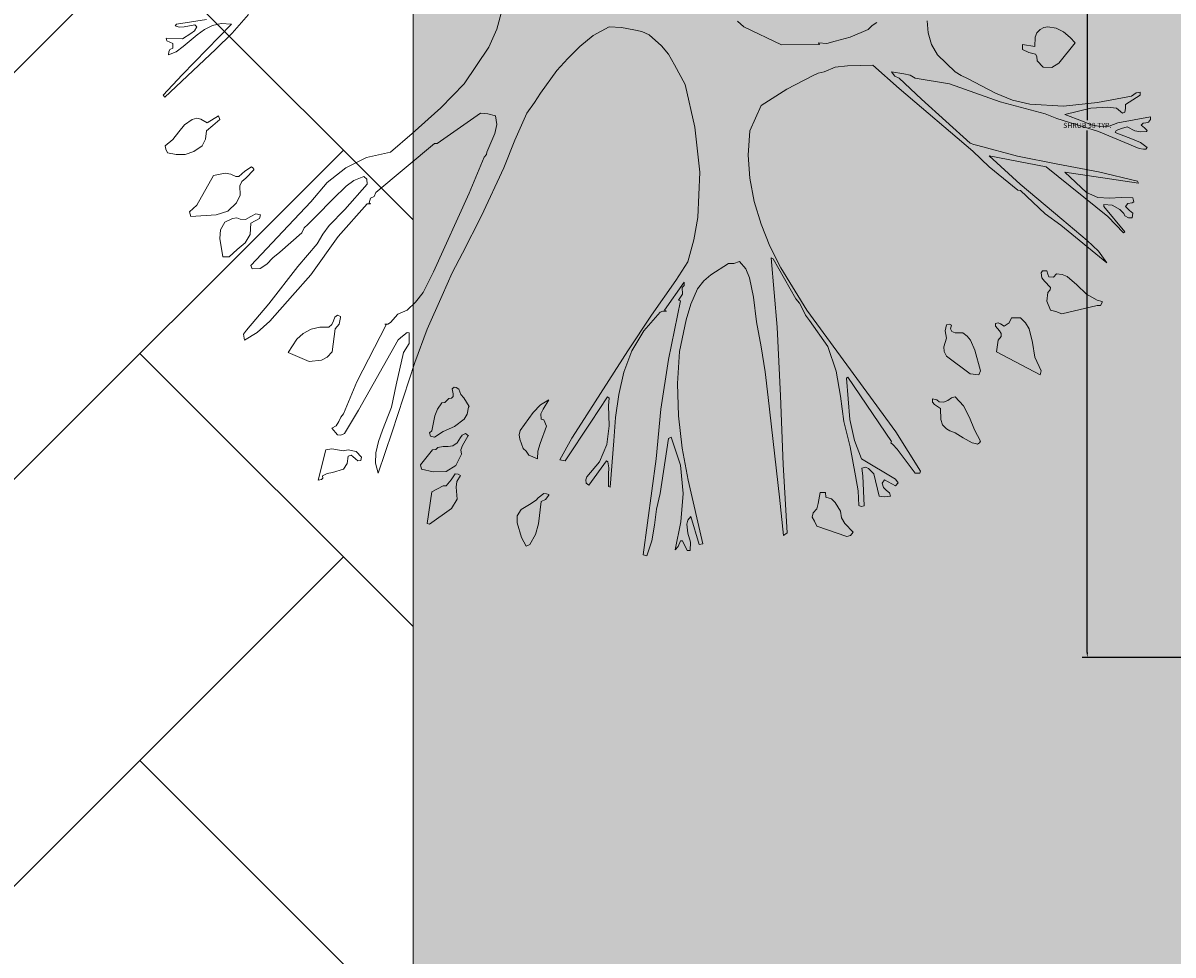
# Model space of a CAD drawing. Units: inches. Extents: x 84 to 1044, y -280 to 906.
# Tile 9 of 105: x 441 to 482, y -79 to -46. Entities that reach past the tile are written whole.
import ezdxf

# ---------------------------------------------------------------- set-up
doc = ezdxf.new("R2010")
doc.units = ezdxf.units.IN
for name, color, linetype, lineweight in [('A-ANNO-DIMS', 2, 'Continuous', 18), ('L-HRDS', 32, 'Continuous', 18), ('L-PLNT', 114, 'Continuous', 15)]:
    doc.layers.add(name, color=color, linetype=linetype, lineweight=lineweight)
doc.layers.add('L-PLNT-PATT', color=9, linetype='Continuous', lineweight=9, true_color=0xafd9aa)
doc.layers.add('L-PRKG-PATT', color=35, linetype='Continuous', lineweight=9, true_color=0x947764)
doc.styles.get("Standard").update_dxf_attribs({"font": 'arial.ttf'})
doc.dimstyles.get("Standard").update_dxf_attribs({"dimtxt": 0.18, "dimasz": 0.18, "dimexe": 0.18, "dimexo": 0.0625, "dimgap": 0.09, "dimtad": 0, "dimtih": 1, "dimtoh": 1, "dimdec": 4, "dimzin": 0, "dimdsep": 46, "dimtxsty": 'Standard', "dimcen": 0.09, "dimadec": 0, "dimazin": 0, "dimtfac": 1, "dimtdec": 4, "dimtofl": 0, "dimtmove": 0, "dimatfit": 3, "dimfxl": 1, "dimtolj": 1, "dimtzin": 0, "dimarcsym": 0})

# ---------------------------------------------------------------- blocks, each defined once
blk = doc.blocks.new('A$C37E508DF')
for p, q in [((0.9287, 0.7825), (0.936, 0.7542)), ((1.3151, 0.7487), (1.2919, 0.7752)), ((0.1351, 0.7559), (0.1471, 0.7577)), ((0.1471, 0.7577), (0.1527, 0.7568)), ((0.3186, 0.7491), (0.3199, 0.7662)), ((0.3919, 0.7641), (0.3988, 0.7598)), ((0.3988, 0.7598), (0.4043, 0.7538)), ((0.5287, 0.7319), (0.5823, 0.7577)), ((0.5823, 0.7577), (0.5913, 0.7658)), ((0.7752, 0.7577), (0.7577, 0.7568)), ((0.798, 0.7452), (0.7752, 0.7577)), ((1.3309, 0.7624), (1.3164, 0.7615)), ((1.3164, 0.7615), (1.3871, 0.6891)), ((1.3434, 0.7598), (1.3309, 0.7624)), ((1.355, 0.7538), (1.3434, 0.7598)), ((1.352, 0.7684), (1.3948, 0.7615)), ((1.3687, 0.7607), (1.3657, 0.7577)), ((1.3657, 0.7577), (1.3691, 0.7521)), ((1.3841, 0.7577), (1.3687, 0.7607)), ((1.3914, 0.7572), (1.3841, 0.7577)), ((1.397, 0.759), (1.3914, 0.7572)), ((1.3948, 0.7615), (1.397, 0.759)), ((0.1081, 0.7349), (0.1153, 0.7427)), ((0.1153, 0.7427), (0.1244, 0.7504)), ((0.1244, 0.7504), (0.1351, 0.7559)), ((0.1527, 0.7568), (0.1578, 0.7538)), ((0.1578, 0.7538), (0.1629, 0.7491)), ((0.1629, 0.7491), (0.1651, 0.7431)), ((0.1651, 0.7431), (0.1655, 0.7298)), ((0.3139, 0.7324), (0.3186, 0.7491)), ((0.4043, 0.7538), (0.4301, 0.7431)), ((0.4301, 0.7431), (0.4515, 0.7371)), ((0.7182, 0.7461), (0.7002, 0.7307)), ((0.7285, 0.7512), (0.7182, 0.7461)), ((0.7401, 0.7534), (0.7285, 0.7512)), ((0.7577, 0.7568), (0.7401, 0.7534)), ((0.8173, 0.7298), (0.798, 0.7452)), ((0.936, 0.7542), (0.9476, 0.7285)), ((1.3391, 0.7255), (1.3151, 0.7487)), ((1.3653, 0.7461), (1.355, 0.7538)), ((1.3854, 0.7294), (1.3653, 0.7461)), ((1.3691, 0.7521), (1.3743, 0.7482)), ((1.3743, 0.7482), (1.3863, 0.7405)), ((1.3863, 0.7405), (1.4099, 0.7414)), ((1.4099, 0.7414), (1.4086, 0.7375)), ((0.1312, 0.7058), (0.1081, 0.7349)), ((0.1655, 0.7298), (0.1831, 0.7324)), ((0.1831, 0.7255), (0.1741, 0.7208)), ((0.1831, 0.7324), (0.1831, 0.7255)), ((0.3049, 0.7178), (0.3139, 0.7324)), ((0.4515, 0.7371), (0.4635, 0.7341)), ((0.4635, 0.7341), (0.4755, 0.7349)), ((0.4755, 0.7349), (0.4742, 0.7324)), ((0.4742, 0.7324), (0.5287, 0.7319)), ((0.7002, 0.7307), (0.6903, 0.7186)), ((0.8344, 0.7122), (0.8173, 0.7298)), ((0.9476, 0.7285), (0.9828, 0.6762)), ((1.4116, 0.6569), (1.3391, 0.7255)), ((1.3953, 0.7221), (1.3854, 0.7294)), ((1.4086, 0.7375), (1.4004, 0.7337)), ((1.4004, 0.7337), (1.4004, 0.7272)), ((1.4004, 0.7272), (1.4047, 0.7255)), ((1.4047, 0.7255), (1.406, 0.7221)), ((0.1621, 0.7092), (0.1539, 0.7002)), ((0.1629, 0.7152), (0.1621, 0.7092)), ((0.1646, 0.7186), (0.1629, 0.7152)), ((0.1741, 0.7208), (0.1646, 0.7186)), ((0.28, 0.6933), (0.3049, 0.7178)), ((0.6903, 0.7186), (0.6818, 0.7032)), ((0.8503, 0.6951), (0.8344, 0.7122)), ((1.4064, 0.7178), (1.3953, 0.7221)), ((1.406, 0.7221), (1.4064, 0.7178)), ((0.1415, 0.6994), (0.1312, 0.7058)), ((0.1539, 0.7002), (0.1415, 0.6994)), ((0.271, 0.6882), (0.28, 0.6933)), ((0.3709, 0.6933), (0.3533, 0.6903)), ((0.3975, 0.7028), (0.3598, 0.6693)), ((0.3662, 0.6873), (0.3709, 0.6933)), ((0.4339, 0.7019), (0.3975, 0.7028)), ((0.4515, 0.7002), (0.4339, 0.7019)), ((0.4674, 0.6933), (0.4515, 0.7002)), ((0.476, 0.6912), (0.4674, 0.6933)), ((0.6818, 0.7032), (0.6667, 0.6749)), ((0.8739, 0.6629), (0.8503, 0.6951)), ((0.2877, 0.6762), (0.2152, 0.6505)), ((0.2221, 0.6625), (0.262, 0.6839)), ((0.262, 0.6839), (0.271, 0.6882)), ((0.337, 0.6843), (0.2877, 0.6762)), ((0.328, 0.6543), (0.3598, 0.6843)), ((0.3443, 0.6886), (0.337, 0.6843)), ((0.3533, 0.6903), (0.3443, 0.6886)), ((0.3598, 0.6843), (0.3662, 0.6873)), ((0.4832, 0.6878), (0.476, 0.6912)), ((0.521, 0.6685), (0.4832, 0.6878)), ((0.9828, 0.6762), (1.0162, 0.6415)), ((1.3871, 0.6891), (1.4141, 0.6599)), ((0.0146, 0.6599), (0.0146, 0.6642)), ((0.0146, 0.6642), (0.0206, 0.6633)), ((0.036, 0.6466), (0.0146, 0.6599)), ((0.0206, 0.6633), (0.0274, 0.6586)), ((0.1977, 0.6526), (0.2221, 0.6625)), ((0.3598, 0.6693), (0.2543, 0.5797)), ((0.5578, 0.6449), (0.521, 0.6685)), ((0.6667, 0.6749), (0.6526, 0.614)), ((0.8824, 0.6492), (0.8739, 0.6629)), ((1.4141, 0.6599), (1.4116, 0.6569)), ((0.0274, 0.6586), (0.0759, 0.6492)), ((0.0356, 0.6406), (0.036, 0.6466)), ((0.0609, 0.6428), (0.0489, 0.641)), ((0.0853, 0.641), (0.0609, 0.6428)), ((0.0759, 0.6492), (0.1244, 0.644)), ((0.1244, 0.644), (0.1728, 0.647)), ((0.2152, 0.6505), (0.1509, 0.6333)), ((0.1728, 0.647), (0.1977, 0.6526)), ((0.2581, 0.5913), (0.328, 0.6543)), ((0.5737, 0.6089), (0.5578, 0.6449)), ((0.8932, 0.6342), (0.8824, 0.6492)), ((0, 0.629), (0.0467, 0.62)), ((0, 0.6252), (0, 0.629)), ((0.0369, 0.6355), (0.0356, 0.6406)), ((0.0399, 0.6342), (0.0369, 0.6355)), ((0.0489, 0.641), (0.0399, 0.6342)), ((0.1226, 0.632), (0.0853, 0.641)), ((0.0973, 0.6226), (0.1226, 0.632)), ((0.1342, 0.6265), (0.1175, 0.6213)), ((0.1509, 0.6333), (0.1342, 0.6265)), ((0.9103, 0.5956), (0.8932, 0.6342)), ((0.9382, 0.6303), (0.936, 0.6179)), ((0.9493, 0.6333), (0.9382, 0.6303)), ((0.9596, 0.6342), (0.9493, 0.6333)), ((1.0218, 0.5904), (0.9596, 0.6342)), ((1.0162, 0.6415), (1.0574, 0.605)), ((1.3327, 0.6252), (1.3348, 0.6303)), ((1.3348, 0.6303), (1.3511, 0.62)), ((1.3601, 0.6256), (1.3661, 0.6269)), ((1.3661, 0.6269), (1.3725, 0.6252)), ((0.003, 0.6213), (0, 0.6252)), ((0.0069, 0.6204), (0.003, 0.6213)), ((0.0047, 0.6093), (0.0086, 0.6132)), ((0.0107, 0.6196), (0.0069, 0.6204)), ((0.0086, 0.6132), (0.0133, 0.617)), ((0.0133, 0.617), (0.0107, 0.6196)), ((0.0334, 0.6145), (0.0223, 0.6089)), ((0.0416, 0.6119), (0.0334, 0.6145)), ((0.0493, 0.6093), (0.0416, 0.6119)), ((0.0467, 0.62), (0.0592, 0.6153)), ((0.0592, 0.6153), (0.072, 0.6149)), ((0.072, 0.6149), (0.0849, 0.6175)), ((0.1175, 0.6213), (0.0746, 0.6076)), ((0.0849, 0.6175), (0.0973, 0.6226)), ((0.6526, 0.614), (0.6457, 0.5497)), ((0.936, 0.6179), (0.939, 0.605)), ((1.343, 0.6162), (1.3327, 0.6252)), ((1.352, 0.6089), (1.343, 0.6162)), ((1.3511, 0.62), (1.3601, 0.6256)), ((1.3725, 0.6252), (1.3837, 0.6175)), ((1.3837, 0.6175), (1.3918, 0.6072)), ((0.0056, 0.6076), (0.0047, 0.6093)), ((0.0141, 0.6072), (0.0056, 0.6076)), ((0.0223, 0.6089), (0.0141, 0.6072)), ((0.0141, 0.5921), (0.0257, 0.5969)), ((0.0746, 0.6076), (0.0163, 0.5836)), ((0.0257, 0.5969), (0.0506, 0.6063)), ((0.0506, 0.6063), (0.0493, 0.6093)), ((0.5763, 0.5741), (0.5737, 0.6089)), ((0.9262, 0.5557), (0.9103, 0.5956)), ((0.939, 0.605), (0.9506, 0.5784)), ((1.0574, 0.605), (1.0883, 0.5784)), ((1.3533, 0.5969), (1.352, 0.6089)), ((1.358, 0.5874), (1.3533, 0.5969)), ((1.3918, 0.6072), (1.4004, 0.5964)), ((1.4004, 0.5964), (1.4111, 0.5874)), ((0.0047, 0.5849), (0.0141, 0.5921)), ((0.0069, 0.5823), (0.0047, 0.5849)), ((0.0099, 0.5823), (0.0069, 0.5823)), ((0.0163, 0.5836), (0.0099, 0.5823)), ((0.1904, 0.5724), (0.2474, 0.5879)), ((0.2543, 0.5797), (0.2311, 0.557)), ((0.2474, 0.5879), (0.253, 0.5892)), ((0.253, 0.5892), (0.2581, 0.5913)), ((0.9506, 0.5784), (0.951, 0.5746)), ((1.0256, 0.5904), (1.0218, 0.5904)), ((1.1097, 0.5205), (1.0256, 0.5904)), ((1.0883, 0.5784), (1.123, 0.5703)), ((1.37, 0.5789), (1.358, 0.5874)), ((1.3824, 0.575), (1.37, 0.5789)), ((1.4077, 0.5771), (1.3953, 0.5746)), ((1.4103, 0.5823), (1.4077, 0.5771)), ((1.4111, 0.5874), (1.4103, 0.5823)), ((0.0746, 0.5501), (0.1325, 0.5608)), ((0.1325, 0.5608), (0.1904, 0.5724)), ((0.2311, 0.5729), (0.1496, 0.557)), ((0.1869, 0.5325), (0.2311, 0.5729)), ((0.5737, 0.5407), (0.5763, 0.5741)), ((0.951, 0.5746), (0.9545, 0.5711)), ((0.9545, 0.5711), (0.9759, 0.5193)), ((1.123, 0.5703), (1.1526, 0.5557)), ((1.3953, 0.5746), (1.3824, 0.575)), ((0.1226, 0.5497), (0.0171, 0.5338)), ((0.0184, 0.5368), (0.0746, 0.5501)), ((0.1496, 0.557), (0.0613, 0.4858)), ((0.0917, 0.5205), (0.1226, 0.5497)), ((0.2311, 0.557), (0.1899, 0.5235)), ((0.6457, 0.5497), (0.6483, 0.4845)), ((0.9583, 0.4871), (0.9262, 0.5557)), ((1.1526, 0.5557), (1.1792, 0.5347)), ((1.2842, 0.554), (1.2855, 0.5557)), ((1.2842, 0.5527), (1.2842, 0.554)), ((1.2958, 0.5407), (1.2842, 0.5527)), ((1.2855, 0.5557), (1.2876, 0.557)), ((1.2876, 0.557), (1.2971, 0.551)), ((1.2971, 0.551), (1.3057, 0.5433)), ((1.3099, 0.5433), (1.3172, 0.5467)), ((1.3172, 0.5467), (1.3254, 0.548)), ((1.3254, 0.548), (1.3421, 0.5446)), ((1.3421, 0.5446), (1.3657, 0.5021)), ((0.0171, 0.5338), (0.0184, 0.5368)), ((0.1269, 0.482), (0.1869, 0.5325)), ((0.5677, 0.5077), (0.5737, 0.5407)), ((1.1226, 0.5394), (1.1221, 0.5325)), ((1.1221, 0.5325), (1.1539, 0.4961)), ((1.1268, 0.5433), (1.1226, 0.5394)), ((1.141, 0.5377), (1.1268, 0.5433)), ((1.1521, 0.5296), (1.141, 0.5377)), ((1.1706, 0.5111), (1.1521, 0.5296)), ((1.1792, 0.5347), (1.2027, 0.5072)), ((1.3014, 0.536), (1.2958, 0.5407)), ((1.3044, 0.53), (1.3014, 0.536)), ((1.3039, 0.5167), (1.3044, 0.53)), ((1.3057, 0.5433), (1.3099, 0.5433)), ((0.024, 0.5072), (0.0253, 0.5128)), ((0.0253, 0.5128), (0.042, 0.5133)), ((0.042, 0.5133), (0.0587, 0.5124)), ((0.0587, 0.5124), (0.0755, 0.5133)), ((0.0755, 0.5133), (0.0917, 0.5205)), ((0.1861, 0.5231), (0.1509, 0.4897)), ((0.1899, 0.5235), (0.1861, 0.5231)), ((0.9759, 0.5193), (1.0269, 0.4069)), ((1.1118, 0.5145), (1.1097, 0.5205)), ((1.117, 0.5124), (1.1118, 0.5145)), ((1.1191, 0.5055), (1.117, 0.5124)), ((1.1955, 0.4858), (1.1706, 0.5111)), ((1.3091, 0.5055), (1.3039, 0.5167)), ((0.0262, 0.5055), (0.024, 0.5072)), ((0.0253, 0.491), (0.03, 0.4948)), ((0.0326, 0.5047), (0.0262, 0.5055)), ((0.03, 0.4948), (0.036, 0.5004)), ((0.036, 0.5004), (0.0326, 0.5047)), ((0.0369, 0.4639), (0.0669, 0.5004)), ((0.0437, 0.4961), (0.0403, 0.4922)), ((0.0549, 0.5021), (0.0437, 0.4961)), ((0.0669, 0.5034), (0.0549, 0.5021)), ((0.0669, 0.5004), (0.0669, 0.5034)), ((0.5578, 0.4751), (0.5677, 0.5077)), ((1.117, 0.5042), (1.1191, 0.5055)), ((1.1217, 0.5042), (1.117, 0.5042)), ((1.1633, 0.4575), (1.1217, 0.5042)), ((1.1539, 0.4961), (1.1762, 0.4729)), ((1.2027, 0.5072), (1.2426, 0.4644)), ((1.3215, 0.4935), (1.3091, 0.5055)), ((1.3657, 0.5021), (1.3764, 0.4927)), ((0.0262, 0.4841), (0.0253, 0.491)), ((0.0317, 0.4841), (0.0262, 0.4841)), ((0.0369, 0.4871), (0.0317, 0.4841)), ((0.0382, 0.4905), (0.0369, 0.4871)), ((0.0403, 0.4922), (0.0382, 0.4905)), ((0.0613, 0.4858), (0.0386, 0.4627)), ((0.0905, 0.4515), (0.1269, 0.482)), ((0.1509, 0.4897), (0.1282, 0.4734)), ((0.6483, 0.4845), (0.6539, 0.4524)), ((0.9853, 0.4335), (0.9583, 0.4871)), ((1.207, 0.4747), (1.1955, 0.4858)), ((1.2748, 0.4884), (1.2812, 0.4897)), ((1.2761, 0.4832), (1.2748, 0.4884)), ((1.2825, 0.4798), (1.2761, 0.4832)), ((1.2812, 0.4897), (1.2885, 0.4862)), ((1.2885, 0.4764), (1.2825, 0.4798)), ((1.2885, 0.4862), (1.2962, 0.4815)), ((1.2962, 0.4815), (1.3039, 0.482)), ((1.3039, 0.482), (1.3087, 0.4841)), ((1.3087, 0.4841), (1.3147, 0.4832)), ((1.3147, 0.4832), (1.3258, 0.4777)), ((1.3382, 0.4884), (1.3215, 0.4935)), ((1.3258, 0.4777), (1.3318, 0.4669)), ((1.3743, 0.4858), (1.3382, 0.4884)), ((1.3764, 0.4927), (1.3743, 0.4858)), ((0.0386, 0.4627), (0.0369, 0.4639)), ((0.1282, 0.4734), (0.0626, 0.4198)), ((0.545, 0.4434), (0.5578, 0.4751)), ((1.1762, 0.4729), (1.1856, 0.4605)), ((1.2122, 0.47), (1.207, 0.4747)), ((1.2156, 0.4627), (1.2122, 0.47)), ((1.2469, 0.4348), (1.2156, 0.4627)), ((1.2426, 0.4644), (1.2885, 0.4159)), ((1.2894, 0.4601), (1.2885, 0.4764)), ((1.3318, 0.4669), (1.3331, 0.4545)), ((0.0746, 0.4361), (0.0905, 0.4515)), ((0.6539, 0.4524), (0.6625, 0.4211)), ((1.2027, 0.4026), (1.1633, 0.4575)), ((1.1856, 0.4605), (1.1933, 0.4468)), ((1.1933, 0.4468), (1.2212, 0.4146)), ((1.2967, 0.4485), (1.2894, 0.4601)), ((1.3082, 0.4386), (1.2967, 0.4485)), ((1.3331, 0.4545), (1.3284, 0.4284)), ((0.0626, 0.4198), (0.0746, 0.4361)), ((0.5295, 0.4125), (0.545, 0.4434)), ((1.0003, 0.4052), (0.9853, 0.4335)), ((1.2568, 0.4266), (1.2469, 0.4348)), ((1.3198, 0.4284), (1.3082, 0.4386)), ((1.3284, 0.4284), (1.3198, 0.4284)), ((0.4922, 0.3516), (0.5295, 0.4125)), ((0.5403, 0.4254), (0.5081, 0.3679)), ((0.5347, 0.3276), (0.5433, 0.4266)), ((0.5433, 0.4266), (0.5403, 0.4254)), ((0.5887, 0.4215), (0.5797, 0.4112)), ((0.5969, 0.4189), (0.5887, 0.4215)), ((0.6046, 0.4189), (0.5969, 0.4189)), ((0.6295, 0.4022), (0.6046, 0.4189)), ((0.6625, 0.4211), (0.6796, 0.3945)), ((1.2212, 0.4146), (1.2628, 0.361)), ((1.2658, 0.4176), (1.2568, 0.4266)), ((1.2752, 0.4116), (1.2658, 0.4176)), ((1.2885, 0.4159), (1.2868, 0.4108)), ((0.1055, 0.388), (0.1192, 0.4001)), ((0.1192, 0.4001), (0.1265, 0.4031)), ((0.1265, 0.4031), (0.1346, 0.4039)), ((0.1346, 0.4039), (0.1389, 0.3992)), ((0.1389, 0.3992), (0.1458, 0.3996)), ((0.1458, 0.3996), (0.1471, 0.4035)), ((0.1471, 0.4035), (0.1484, 0.4082)), ((0.1484, 0.4082), (0.1548, 0.4082)), ((0.1556, 0.3983), (0.1518, 0.3932)), ((0.1548, 0.4082), (0.1565, 0.4052)), ((0.1565, 0.4052), (0.1556, 0.3983)), ((0.5741, 0.3983), (0.5686, 0.3705)), ((0.5797, 0.4112), (0.5741, 0.3983)), ((0.6397, 0.3936), (0.6295, 0.4022)), ((1.0145, 0.373), (1.0003, 0.4052)), ((1.0269, 0.4069), (1.0419, 0.3769)), ((1.2289, 0.373), (1.2027, 0.4026)), ((1.2868, 0.4108), (1.2752, 0.4116)), ((0.0917, 0.3748), (0.1055, 0.388)), ((0.1518, 0.3932), (0.1432, 0.3842)), ((0.1432, 0.3842), (0.1436, 0.3808)), ((0.1436, 0.3808), (0.1471, 0.3769)), ((0.6487, 0.3825), (0.6397, 0.3936)), ((0.6582, 0.3602), (0.6487, 0.3825)), ((0.6959, 0.352), (0.668, 0.3919)), ((0.668, 0.3919), (0.668, 0.3872)), ((0.668, 0.3872), (0.6706, 0.3842)), ((0.6706, 0.3842), (0.6702, 0.3748)), ((0.6796, 0.3945), (0.7148, 0.3447)), ((0.069, 0.364), (0.0763, 0.3662)), ((0.069, 0.3627), (0.069, 0.364)), ((0.0716, 0.3585), (0.069, 0.3627)), ((0.0763, 0.3662), (0.0917, 0.3748)), ((0.1484, 0.3649), (0.1432, 0.352)), ((0.1471, 0.3769), (0.1484, 0.3649)), ((0.5081, 0.3679), (0.5025, 0.3619)), ((0.5686, 0.3705), (0.5643, 0.3349)), ((0.6702, 0.3748), (0.6762, 0.3662)), ((0.6762, 0.3662), (0.6732, 0.3653)), ((0.6732, 0.3653), (0.6903, 0.2813)), ((1.0359, 0.3246), (1.0145, 0.373)), ((1.0419, 0.3769), (1.0527, 0.3632)), ((1.0527, 0.3632), (1.0647, 0.352)), ((1.2615, 0.3362), (1.2289, 0.373)), ((0.0763, 0.3585), (0.0716, 0.3585)), ((0.1269, 0.3464), (0.0763, 0.3585)), ((0.1355, 0.3499), (0.1269, 0.3464)), ((0.1432, 0.352), (0.1355, 0.3499)), ((0.4065, 0.2345), (0.4922, 0.3516)), ((0.4982, 0.3537), (0.4939, 0.3447)), ((0.5025, 0.3619), (0.4982, 0.3537)), ((0.665, 0.3379), (0.6582, 0.3602)), ((0.6933, 0.3503), (0.6959, 0.352)), ((0.6985, 0.3503), (0.6933, 0.3503)), ((0.7023, 0.349), (0.6985, 0.3503)), ((0.7259, 0.3224), (0.7023, 0.349)), ((1.0647, 0.352), (1.078, 0.346)), ((1.078, 0.346), (1.0883, 0.334)), ((1.2628, 0.361), (1.2949, 0.3233)), ((0.1737, 0.325), (0.1788, 0.3336)), ((0.1788, 0.3336), (0.1861, 0.3409)), ((0.1861, 0.3409), (0.199, 0.3409)), ((0.199, 0.3409), (0.2024, 0.3336)), ((0.2024, 0.3336), (0.2097, 0.3289)), ((0.2097, 0.3289), (0.2148, 0.3323)), ((0.2148, 0.3323), (0.2182, 0.3336)), ((0.2182, 0.3336), (0.2221, 0.3327)), ((0.2221, 0.3327), (0.2221, 0.3289)), ((0.2851, 0.3302), (0.2877, 0.3319)), ((0.2864, 0.325), (0.2851, 0.3302)), ((0.2877, 0.3319), (0.292, 0.3306)), ((0.292, 0.3306), (0.2941, 0.322)), ((0.4884, 0.337), (0.4622, 0.2997)), ((0.4939, 0.3447), (0.4884, 0.337)), ((0.5643, 0.3349), (0.5578, 0.2993)), ((0.6745, 0.2924), (0.665, 0.3379)), ((0.7148, 0.3447), (0.7487, 0.2937)), ((1.0883, 0.334), (1.0921, 0.3319)), ((1.0921, 0.3319), (1.0968, 0.3319)), ((1.0968, 0.3319), (1.0947, 0.3306)), ((1.0947, 0.3306), (1.1367, 0.2491)), ((1.1599, 0.3426), (1.1646, 0.3447)), ((1.1599, 0.3413), (1.1599, 0.3426)), ((1.162, 0.3319), (1.1599, 0.3413)), ((1.1676, 0.325), (1.162, 0.3319)), ((1.1646, 0.3447), (1.168, 0.3417)), ((1.168, 0.3417), (1.1702, 0.3366)), ((1.1702, 0.3366), (1.1727, 0.3314)), ((1.1727, 0.3314), (1.177, 0.3276)), ((1.2795, 0.3199), (1.2615, 0.3362)), ((0.1689, 0.3053), (0.1737, 0.325)), ((0.2161, 0.3224), (0.214, 0.3186)), ((0.214, 0.3186), (0.214, 0.3139)), ((0.214, 0.3139), (0.2182, 0.3087)), ((0.2221, 0.3289), (0.2161, 0.3224)), ((0.2577, 0.3087), (0.2624, 0.3147)), ((0.2624, 0.3147), (0.2689, 0.3194)), ((0.2689, 0.3194), (0.2796, 0.3194)), ((0.2796, 0.3194), (0.2847, 0.3211)), ((0.2847, 0.3211), (0.2864, 0.325)), ((0.2941, 0.322), (0.292, 0.3117)), ((0.53, 0.229), (0.5347, 0.3276)), ((0.7427, 0.2937), (0.7259, 0.3224)), ((1.0535, 0.2766), (1.0359, 0.3246)), ((1.0647, 0.3199), (1.0617, 0.3194)), ((1.0617, 0.3194), (1.0617, 0.304)), ((1.0711, 0.3147), (1.0647, 0.3199)), ((1.0775, 0.3092), (1.0711, 0.3147)), ((1.1719, 0.292), (1.1676, 0.325)), ((1.177, 0.3276), (1.1895, 0.3276)), ((1.1895, 0.3276), (1.2019, 0.3246)), ((1.2019, 0.3246), (1.2135, 0.3186)), ((1.2135, 0.3186), (1.2225, 0.3104)), ((1.2975, 0.3087), (1.2795, 0.3199)), ((1.2949, 0.3233), (1.2988, 0.3173)), ((1.2988, 0.3173), (1.2975, 0.3087)), ((0.1655, 0.2843), (0.1689, 0.3053)), ((0.2182, 0.3087), (0.2204, 0.292)), ((0.2517, 0.2946), (0.2577, 0.3087)), ((0.292, 0.3117), (0.2959, 0.2993)), ((0.2959, 0.2993), (0.2954, 0.2928)), ((0.4622, 0.2997), (0.4502, 0.2645)), ((0.5578, 0.2993), (0.5518, 0.2633)), ((1.0617, 0.304), (1.0698, 0.2911)), ((1.1341, 0.2084), (1.0775, 0.3092)), ((1.2225, 0.3104), (1.2349, 0.2911)), ((0.1565, 0.265), (0.1655, 0.2843)), ((0.2204, 0.292), (0.1578, 0.259)), ((0.2436, 0.265), (0.2517, 0.2946)), ((0.292, 0.286), (0.2581, 0.2607)), ((0.2954, 0.2928), (0.292, 0.286)), ((0.6775, 0.2465), (0.6745, 0.2924)), ((0.6903, 0.2813), (0.7015, 0.2101)), ((0.7542, 0.2628), (0.7427, 0.2937)), ((0.7487, 0.2937), (0.8151, 0.1899)), ((1.0698, 0.2911), (1.0805, 0.2448)), ((1.1792, 0.2847), (1.1719, 0.292)), ((1.1873, 0.28), (1.1792, 0.2847)), ((1.2349, 0.2911), (1.2049, 0.2783)), ((0.1578, 0.259), (0.1565, 0.265)), ((0.2461, 0.259), (0.2436, 0.265)), ((0.4502, 0.2645), (0.4438, 0.2285)), ((1.0861, 0.1775), (1.0535, 0.2766)), ((1.2049, 0.2783), (1.1873, 0.28)), ((0.2581, 0.2607), (0.2461, 0.259)), ((0.4335, 0.2556), (0.3709, 0.1634)), ((0.4305, 0.1951), (0.4352, 0.2543)), ((0.4352, 0.2543), (0.4335, 0.2556)), ((0.5518, 0.2633), (0.5475, 0.2268)), ((0.7615, 0.2311), (0.7542, 0.2628)), ((1.1367, 0.2491), (1.1556, 0.2032)), ((0.3649, 0.1775), (0.4065, 0.2345)), ((0.6758, 0.2002), (0.6775, 0.2465)), ((0.7662, 0.1981), (0.7615, 0.2311)), ((0.9836, 0.226), (0.9879, 0.2311)), ((0.9879, 0.2311), (0.9905, 0.2384)), ((0.9905, 0.2384), (0.9943, 0.241)), ((0.9943, 0.241), (0.9973, 0.2414)), ((0.9973, 0.2414), (1.0003, 0.2393)), ((1.0003, 0.2393), (0.9986, 0.232)), ((0.9986, 0.232), (0.9986, 0.2281)), ((1.0805, 0.2448), (1.087, 0.2127)), ((0.2594, 0.1981), (0.268, 0.2148)), ((0.268, 0.2148), (0.28, 0.2277)), ((0.28, 0.2277), (0.2851, 0.226)), ((0.2851, 0.226), (0.2903, 0.2225)), ((0.2903, 0.2225), (0.2963, 0.22)), ((0.2963, 0.22), (0.3027, 0.2204)), ((0.3096, 0.2165), (0.301, 0.211)), ((0.3027, 0.2204), (0.3061, 0.2234)), ((0.3061, 0.2234), (0.3122, 0.2247)), ((0.3122, 0.22), (0.3096, 0.2165)), ((0.3122, 0.2247), (0.3122, 0.22)), ((0.4438, 0.2285), (0.4391, 0.1921)), ((0.5261, 0.1308), (0.53, 0.229)), ((0.5475, 0.2268), (0.5313, 0.084)), ((0.7778, 0.2277), (0.7752, 0.2255)), ((0.7752, 0.2255), (0.7761, 0.2152)), ((0.7761, 0.2152), (0.7752, 0.1861)), ((0.8018, 0.1912), (0.7778, 0.2277)), ((0.8619, 0.2234), (0.8739, 0.2161)), ((0.87, 0.2101), (0.8619, 0.2234)), ((0.8739, 0.2161), (0.8841, 0.2054)), ((0.9759, 0.214), (0.9836, 0.226)), ((0.9986, 0.2281), (1.0012, 0.2255)), ((1.0012, 0.2255), (1.0051, 0.2251)), ((1.0051, 0.2251), (1.0076, 0.2225)), ((1.0076, 0.2225), (1.0106, 0.2195)), ((1.0106, 0.2195), (1.0149, 0.2191)), ((1.0149, 0.2191), (1.0214, 0.2101)), ((0.2521, 0.1805), (0.2594, 0.1981)), ((0.301, 0.211), (0.3002, 0.1951)), ((0.6706, 0.1539), (0.6758, 0.2002)), ((0.7015, 0.2101), (0.7079, 0.1389)), ((0.7688, 0.1646), (0.7662, 0.1981)), ((0.8734, 0.2032), (0.87, 0.2101)), ((0.8726, 0.1955), (0.8734, 0.2032)), ((0.8841, 0.2054), (0.9026, 0.1792)), ((0.9768, 0.2127), (0.9759, 0.214)), ((0.9789, 0.2028), (0.9768, 0.2127)), ((0.9832, 0.1955), (0.9789, 0.2028)), ((1.0214, 0.2101), (1.0252, 0.2002)), ((1.0252, 0.2002), (1.0295, 0.1788)), ((1.087, 0.2127), (1.0998, 0.1797)), ((1.1543, 0.1749), (1.1341, 0.2084)), ((1.1556, 0.2032), (1.1594, 0.1985)), ((1.1594, 0.1985), (1.1624, 0.1921)), ((0.292, 0.1818), (0.2873, 0.1788)), ((0.298, 0.1874), (0.292, 0.1818)), ((0.3002, 0.1951), (0.298, 0.1874)), ((0.4241, 0.1651), (0.4305, 0.1951)), ((0.4391, 0.1921), (0.4301, 0.1561)), ((0.7752, 0.1861), (0.7787, 0.1591)), ((0.8383, 0.1359), (0.8018, 0.1912)), ((0.8151, 0.1899), (0.8288, 0.1685)), ((0.8649, 0.1857), (0.8687, 0.1947)), ((0.8743, 0.1608), (0.8649, 0.1857)), ((0.8687, 0.1947), (0.8726, 0.1955)), ((0.9969, 0.1852), (0.9832, 0.1955)), ((1.0132, 0.1779), (0.9969, 0.1852)), ((1.1624, 0.1921), (1.1663, 0.1861)), ((1.1727, 0.1827), (1.1646, 0.1732)), ((1.1663, 0.1861), (1.1727, 0.1827)), ((0.2436, 0.1642), (0.2521, 0.1805)), ((0.2684, 0.1689), (0.2556, 0.1616)), ((0.28, 0.1762), (0.2684, 0.1689)), ((0.2873, 0.1788), (0.28, 0.1762)), ((0.3293, 0.1213), (0.3649, 0.1775)), ((0.4138, 0.1389), (0.4241, 0.1651)), ((0.6865, 0.1698), (0.6732, 0.1295)), ((0.6903, 0.1681), (0.6865, 0.1698)), ((0.7023, 0.0892), (0.6903, 0.1681)), ((0.8288, 0.1685), (0.846, 0.1376)), ((0.9035, 0.1668), (0.8983, 0.1535)), ((0.9026, 0.1792), (0.9043, 0.1732)), ((0.9043, 0.1732), (0.9035, 0.1668)), ((0.9768, 0.1719), (0.9811, 0.1749)), ((0.9776, 0.1711), (0.9768, 0.1719)), ((0.9853, 0.1578), (0.9776, 0.1711)), ((0.9811, 0.1749), (0.9858, 0.1728)), ((0.9858, 0.1728), (0.9884, 0.1694)), ((0.9884, 0.1694), (0.9931, 0.1616)), ((1.0256, 0.1698), (1.0132, 0.1779)), ((1.0312, 0.1711), (1.0256, 0.1698)), ((1.0295, 0.1788), (1.0325, 0.1762)), ((1.0325, 0.1762), (1.0312, 0.1711)), ((1.1063, 0.1183), (1.0861, 0.1775)), ((1.0998, 0.1797), (1.1058, 0.1634)), ((1.1594, 0.1728), (1.1543, 0.1749)), ((1.1646, 0.1732), (1.1594, 0.1728)), ((0.2448, 0.1616), (0.2436, 0.1642)), ((0.2478, 0.1599), (0.2448, 0.1616)), ((0.2508, 0.1608), (0.2478, 0.1599)), ((0.2556, 0.1616), (0.2508, 0.1608)), ((0.3628, 0.1526), (0.337, 0.1183)), ((0.3692, 0.1591), (0.3628, 0.1526)), ((0.3718, 0.1616), (0.3692, 0.1591)), ((0.3709, 0.1634), (0.3718, 0.1616)), ((0.4301, 0.1561), (0.4224, 0.1145)), ((0.662, 0.108), (0.6706, 0.1539)), ((0.774, 0.0982), (0.7688, 0.1646)), ((0.7787, 0.1591), (0.789, 0.1346)), ((0.8777, 0.1496), (0.8743, 0.1608)), ((0.8781, 0.1389), (0.8777, 0.1496)), ((0.894, 0.1496), (0.8902, 0.1441)), ((0.8983, 0.1535), (0.894, 0.1496)), ((0.9879, 0.1518), (0.9853, 0.1578)), ((0.9866, 0.1453), (0.9879, 0.1518)), ((0.9931, 0.1616), (0.9991, 0.1574)), ((0.9991, 0.1574), (1.0059, 0.1565)), ((1.0059, 0.1565), (1.0132, 0.1565)), ((1.0132, 0.1565), (1.0205, 0.1548)), ((1.0205, 0.1548), (1.0235, 0.1522)), ((1.0235, 0.1522), (1.0282, 0.1518)), ((1.0282, 0.1518), (1.0454, 0.1303)), ((1.1058, 0.1634), (1.1097, 0.1475)), ((1.1298, 0.1411), (1.1376, 0.1492)), ((1.1376, 0.1492), (1.1491, 0.1518)), ((1.1491, 0.1518), (1.1564, 0.1505)), ((1.1564, 0.1505), (1.1642, 0.1518)), ((1.1642, 0.1518), (1.1727, 0.1531)), ((1.1727, 0.1531), (1.1813, 0.1518)), ((1.1813, 0.1518), (1.192, 0.108)), ((0.3653, 0.1098), (0.4138, 0.1389)), ((0.7079, 0.1389), (0.7268, 0.0013)), ((0.7774, 0.1346), (0.7757, 0.1261)), ((0.7791, 0.1359), (0.7774, 0.1346)), ((0.8044, 0.1012), (0.7791, 0.1359)), ((0.789, 0.1346), (0.8074, 0.1132)), ((0.846, 0.1376), (0.8383, 0.1359)), ((0.8846, 0.1419), (0.8781, 0.1389)), ((0.8902, 0.1441), (0.8846, 0.1419)), ((0.9948, 0.1291), (0.9866, 0.1453)), ((1.1101, 0.1325), (1.1063, 0.1183)), ((1.1097, 0.1475), (1.1101, 0.1325)), ((1.1311, 0.1364), (1.1298, 0.1411)), ((1.1354, 0.1359), (1.1311, 0.1364)), ((1.1384, 0.1389), (1.1354, 0.1359)), ((1.1423, 0.1423), (1.1384, 0.1389)), ((1.1449, 0.1441), (1.1423, 0.1423)), ((1.1491, 0.1428), (1.1449, 0.1441)), ((1.1504, 0.132), (1.1491, 0.1428)), ((1.1556, 0.1239), (1.1504, 0.132)), ((0.3306, 0.1183), (0.3293, 0.1213)), ((0.337, 0.1183), (0.3306, 0.1183)), ((0.3962, 0.1175), (0.3885, 0.0853)), ((0.4039, 0.1248), (0.3962, 0.1175)), ((0.4082, 0.1269), (0.4039, 0.1248)), ((0.4134, 0.1256), (0.4082, 0.1269)), ((0.4121, 0.1145), (0.4134, 0.1256)), ((0.5205, 0.033), (0.5261, 0.1308)), ((0.6732, 0.1295), (0.6693, 0.0892)), ((0.7757, 0.1261), (0.7761, 0.117)), ((0.7761, 0.117), (0.7761, 0.099)), ((0.9884, 0.1149), (0.9918, 0.117)), ((0.9918, 0.117), (0.9961, 0.1175)), ((1.0089, 0.1205), (0.9948, 0.1291)), ((0.9961, 0.1175), (1.0016, 0.1085)), ((1.0274, 0.12), (1.0089, 0.1205)), ((1.0441, 0.1239), (1.0274, 0.12)), ((1.0454, 0.1303), (1.0441, 0.1239)), ((1.1714, 0.1192), (1.1556, 0.1239)), ((1.1792, 0.1179), (1.1714, 0.1192)), ((1.186, 0.1145), (1.1792, 0.1179)), ((0.3615, 0.1042), (0.3653, 0.1098)), ((0.3653, 0.0999), (0.3615, 0.1042)), ((0.3812, 0.1089), (0.3653, 0.0999)), ((0.3842, 0.1037), (0.3812, 0.1089)), ((0.3825, 0.0978), (0.3842, 0.1037)), ((0.4099, 0.0716), (0.4121, 0.1145)), ((0.4224, 0.1145), (0.4189, 0.093)), ((0.641, 0.0172), (0.662, 0.108)), ((0.7761, 0.099), (0.774, 0.0982)), ((0.8083, 0.1037), (0.8044, 0.1012)), ((0.8074, 0.1132), (0.8087, 0.1089)), ((0.8087, 0.1089), (0.8083, 0.1037)), ((0.9935, 0.1063), (0.9884, 0.1149)), ((0.9943, 0.0982), (0.9935, 0.1063)), ((1.0016, 0.1085), (1.0089, 0.0999)), ((1.0089, 0.0999), (1.0132, 0.0999)), ((1.0132, 0.0999), (1.0295, 0.0917)), ((1.1856, 0.111), (1.186, 0.1145)), ((1.1873, 0.1093), (1.1856, 0.111)), ((1.192, 0.108), (1.1873, 0.1093)), ((0.3722, 0.0853), (0.3739, 0.09)), ((0.3808, 0.0845), (0.3722, 0.0853)), ((0.3739, 0.09), (0.3782, 0.0935)), ((0.3782, 0.0935), (0.3825, 0.0978)), ((0.3885, 0.0853), (0.3808, 0.0845)), ((0.4189, 0.093), (0.4176, 0.072)), ((0.4571, 0.0815), (0.4648, 0.084)), ((0.4648, 0.084), (0.4657, 0.0905)), ((0.4657, 0.0905), (0.473, 0.0905)), ((0.473, 0.0905), (0.476, 0.0746)), ((0.5313, 0.084), (0.5257, 0.0291)), ((0.6693, 0.0892), (0.6728, 0.0484)), ((0.7075, 0.0665), (0.7023, 0.0892)), ((0.8619, 0.0875), (0.8649, 0.0887)), ((0.8619, 0.0866), (0.8619, 0.0875)), ((0.8666, 0.0806), (0.8619, 0.0866)), ((0.8649, 0.0887), (0.8691, 0.0892)), ((0.8691, 0.0892), (0.8769, 0.0827)), ((0.8769, 0.0827), (0.8799, 0.0797)), ((0.9931, 0.081), (0.9943, 0.0982)), ((1.0295, 0.0917), (1.0359, 0.0463)), ((0.4142, 0.0707), (0.4099, 0.0716)), ((0.4176, 0.072), (0.4142, 0.0707)), ((0.4442, 0.0639), (0.4515, 0.0763)), ((0.4515, 0.0763), (0.4571, 0.0815)), ((0.476, 0.0746), (0.4777, 0.0673)), ((0.4777, 0.0673), (0.4832, 0.0613)), ((0.7105, 0.0437), (0.7075, 0.0665)), ((0.8726, 0.0776), (0.8666, 0.0806)), ((0.8764, 0.0459), (0.8726, 0.0776)), ((0.8799, 0.0797), (0.8893, 0.0733)), ((0.8893, 0.0733), (0.9013, 0.066)), ((0.9013, 0.066), (0.9069, 0.057)), ((1.0012, 0.0677), (0.9931, 0.081)), ((1.0325, 0.0454), (1.0012, 0.0677)), ((0.4378, 0.0463), (0.4425, 0.0544)), ((0.4425, 0.0544), (0.4442, 0.0639)), ((0.4845, 0.0553), (0.4811, 0.0493)), ((0.4832, 0.0613), (0.4845, 0.0553)), ((0.6582, 0.0562), (0.6466, 0.0159)), ((0.6625, 0.051), (0.6582, 0.0562)), ((0.6642, 0.045), (0.6625, 0.051)), ((0.9069, 0.057), (0.9069, 0.0471)), ((0.4258, 0.0339), (0.4378, 0.0463)), ((0.4296, 0.0291), (0.4258, 0.0339)), ((0.4777, 0.0424), (0.4348, 0.0274)), ((0.4811, 0.0493), (0.4777, 0.0424)), ((0.5257, 0.0291), (0.5205, 0.033)), ((0.6625, 0.0321), (0.6642, 0.045)), ((0.6728, 0.0484), (0.6809, 0.0082)), ((0.7144, 0.0214), (0.7105, 0.0437)), ((0.8807, 0.0304), (0.8764, 0.0459)), ((0.9069, 0.0471), (0.9009, 0.0261)), ((1.0359, 0.0463), (1.0325, 0.0454)), ((0.4348, 0.0274), (0.4296, 0.0291)), ((0.6466, 0.0159), (0.641, 0.0172)), ((0.659, 0.0193), (0.6625, 0.0321)), ((0.6595, 0.0077), (0.659, 0.0193)), ((0.6702, 0.0214), (0.6637, 0.0077)), ((0.6732, 0.0214), (0.6702, 0.0214)), ((0.6766, 0.0133), (0.6732, 0.0214)), ((0.7216, 0), (0.7144, 0.0214)), ((0.8889, 0.0159), (0.8807, 0.0304)), ((0.9009, 0.0261), (0.894, 0.0137)), ((0.6637, 0.0077), (0.6595, 0.0077)), ((0.6809, 0.0082), (0.6766, 0.0133)), ((0.7268, 0.0013), (0.7216, 0)), ((0.894, 0.0137), (0.8889, 0.0159))]:
    blk.add_line(p, q)
blk = doc.blocks.new('*D28')
at = {"layer": 'A-ANNO-DIMS', "color": 0, "lineweight": -2, "transparency": 16777216}
for p, q in [((484.443, -30.627), (478.69, -30.627)), ((478.87, -30.807), (478.87, -49.227)), ((478.87, -68.013), (478.87, -49.593)), ((484.443, -68.193), (478.69, -68.193))]:
    blk.add_line(p, q, dxfattribs=at)
at = {"layer": 'A-ANNO-DIMS', "color": 0, "transparency": 16777216}
for points in [[(478.84, -30.807), (478.9, -30.807), (478.87, -30.627)], [(478.84, -68.013), (478.9, -68.013), (478.87, -68.193)]]:
    blk.add_solid(points, dxfattribs=at)
at = {"layer": 'Defpoints', "color": 0, "transparency": 16777216}
for p in [(478.87, -30.627), (484.505, -30.627), (484.505, -68.193)]:
    blk.add_point(p, dxfattribs=at)
at = {"layer": 'A-ANNO-DIMS', "color": 0, "transparency": 16777216, "insert": (478.87, -49.41), "char_height": 0.18, "attachment_point": 5}
blk.add_mtext('\\A1;SHRUB 38 TYP.', dxfattribs=at)

msp = doc.modelspace()

# ---------------------------------------------------------------- hatches: boundary and pattern name
at = {"layer": 'L-PLNT-PATT', "transparency": 33554597}
h = msp.add_hatch(color=256, dxfattribs=at)
h.dxf.hatch_style = 1
h.paths.add_polyline_path([(504.574, -40.88), (455.074, -40.88), (455.074, -112.88), (504.574, -112.88)])
at = {"layer": 'L-PRKG-PATT', "transparency": 33554567}
h = msp.add_hatch(dxfattribs=at)
h.set_pattern_fill('AR-HBONE', color=256, scale=0.1)
h.paths.add_polyline_path([(455.074, 31.12), (455.074, 91.12), (455.074, 151.12), (413.127, 151.12), (341.127, 151.12), (290.179, 151.12), (227.179, 151.12), (227.179, 127.12), (143.179, 127.12), (143.179, -112.88), (143.179, -117.88), (455.074, -117.88)])

# ---------------------------------------------------------------- linework, layer by layer
at = {"layer": 'L-HRDS'}
msp.add_line((455.074, 31.12), (455.074, -121.88), dxfattribs=at)

# ---------------------------------------------------------------- block references
at = {"layer": 'L-PLNT', "xscale": -24.64361536662419, "yscale": 24.64361536662419, "zscale": 24.64361536662419}
msp.add_blockref('A$C37E508DF', (481.101, -64.604), dxfattribs=at)

# ---------------------------------------------------------------- dimensions: what is measured, and where the dimension line sits
at = {"layer": 'A-ANNO-DIMS'}
dim = msp.add_linear_dim(base=(478.87, -30.627), p1=(484.505, -68.193), p2=(484.505, -30.627), angle=90, text='SHRUB <> TYP.', dimstyle='Standard', override={"dimdec": 0, "dimlfac": 1, "dimrnd": 0, "dimzin": 0, "dimdsep": 46, "dimlunit": 2}, dxfattribs=at)
dim.commit()
dim.dimension.update_dxf_attribs({"geometry": '*D28', "text_midpoint": (478.87, -49.41)})

doc.saveas('drawing.dxf')
